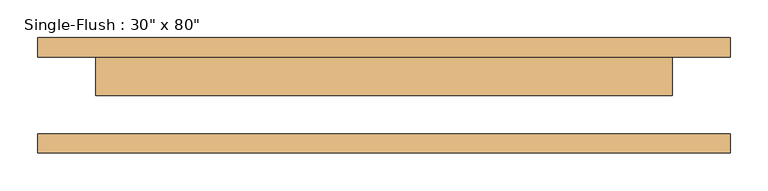
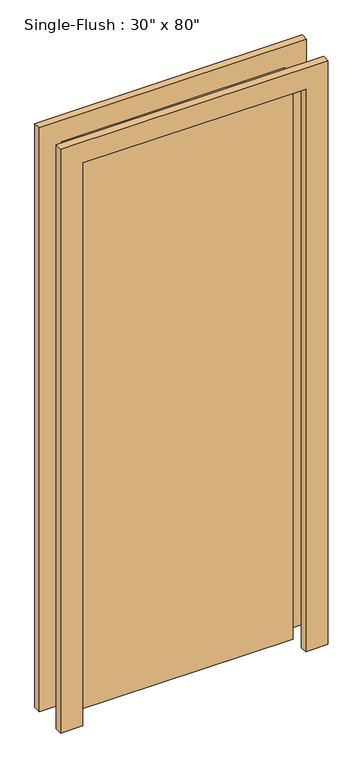
"""IFC4 building model written with IfcOpenShell, lengths in millimetres: door geometry."""

from ifc_helpers import new_model, si_unit, frame, origin, origin_with_axes, place, context, project, spatial, polyline, outline, extrude, source, transform, mapped, element, save


def door_29583826(model_context):
    return source(origin(), model_context, "Body", "SweptSolid", [
        extrude(outline(polyline([(2108.2, -457.2), (0.0, -457.2), (0.0, -381.0), (2032.0, -381.0), (2032.0, 381.0), (0.0, 381.0), (0.0, 457.2), (2108.2, 457.2), (2108.2, -457.2)])), frame((0.0, 50.8, 0.0), z_axis=(0.0, 1.0, 0.0), x_axis=(0.0, 0.0, 1.0)), (0.0, 0.0, 1.0), 25.4),
        extrude(outline(polyline([(2108.2, 457.2), (2108.2, -457.2), (0.0, -457.2), (0.0, -381.0), (2032.0, -381.0), (2032.0, 381.0), (0.0, 381.0), (0.0, 457.2), (2108.2, 457.2)])), frame((0.0, -76.2, 0.0), z_axis=(0.0, 1.0, 0.0), x_axis=(0.0, 0.0, 1.0)), (0.0, 0.0, 1.0), 25.4),
        extrude(outline(polyline([(381.0, 0.0), (-381.0, 0.0), (-381.0, 50.8), (381.0, 50.8), (381.0, 0.0)])), origin_with_axes(), (0.0, 0.0, 1.0), 2032.0),
    ])


if __name__ == "__main__":
    model = new_model("IFC4")
    model_context = context("Model", 3, world=origin())
    ifc_project = project(units=[si_unit("LENGTHUNIT", "METRE", prefix="MILLI")], contexts=[model_context])
    site = spatial("IfcSite", under=ifc_project)
    building = spatial("IfcBuilding", under=site)
    placement = place(None, origin())
    door_shape = door_29583826(model_context)
    element("IfcDoor", 1, ObjectType="Single-Flush : 30\" x 80\"", at=placement, inside=building, context=model_context, shape_type="MappedRepresentation", body=[
        mapped(door_shape, transform((0.0, 0.0, 0.0), x_axis=(1.0, 0.0, 0.0), y_axis=(0.0, 1.0, 0.0), z_axis=(0.0, 0.0, 1.0))),
    ])
    save(model, "model.ifc")

# Revit data of these elements
# Type "Single-Flush : 30\" x 80\""
#   Type Mark = "5"
#   Construction Type Id = "MDOOR"
#   Assembly Code = "C1020"
#   Analytic Construction = "Metal"
#   Thickness = 0' - 2"
#   Heat Transfer Coefficient (U) = 0.651978 BTU/(h·ft²·°F)
#   Height = 6' - 8"
#   Trim Projection Ext = 0' - 1"
#   Trim Projection Int = 0' - 1"
#   Trim Width = 0' - 3"
#   Width = 2' - 6"
#   Define Thermal Properties by = 1
#   Door Material = Door - Panel
#   Frame Material = Door - Frame
#   Visual Light Transmittance = 0
#   Solar Heat Gain Coefficient = 0
#   Function = (empty or 0)
#   Wall Closure = (empty or 0)
# Element 1 (IfcDoor, "Single-Flush : 30\" x 80\"")
#   Materials on its faces: "Door - Frame", "Door - Panel"
# Materials
#   "Door - Panel": class "Wood", colour RGB 210 159 95, transparency 0
#   "Door - Frame": colour RGB 118 70 51, transparency 0
